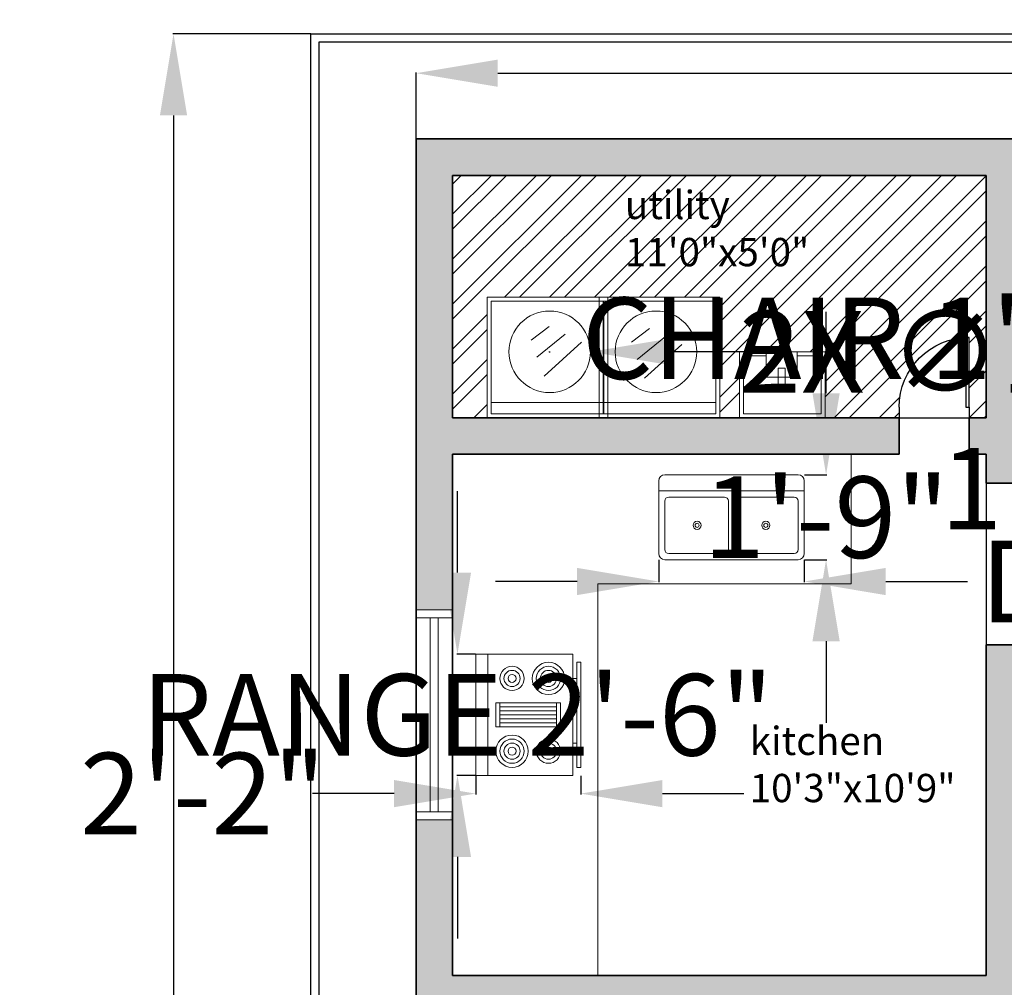
# Model space of a CAD drawing. Units: inches. Extents: x 1202 to 2101, y 998 to 1743.
# Tile 2 of 4: x 1310 to 1553, y 1460 to 1699. Entities that reach past the tile are written whole.
import ezdxf

# ---------------------------------------------------------------- set-up
doc = ezdxf.new("R2010")
doc.units = ezdxf.units.IN
doc.header["$MEASUREMENT"] = 0
for name, color, linetype, lineweight in [('A-ANNO-DIMS', 2, 'Continuous', 18), ('A-AREA-IDEN', 7, 'Continuous', 18), ('A-DOOR', 3, 'Continuous', 25), ('A-EQPM', 8, 'Continuous', 18), ('A-FLOR-CASE', 8, 'Continuous', 18), ('A-FLOR-FIXT', 9, 'Continuous', 18), ('A-FLOR-PATT', 9, 'Continuous', 13), ('A-GLAZ', 4, 'Continuous', 18), ('A-WALL', 7, 'Continuous', 35), ('A-WALL-PATT', 250, 'Continuous', 13), ('C-PROP', 7, 'Continuous', 30)]:
    doc.layers.add(name, color=color, linetype=linetype, lineweight=lineweight)
doc.styles.get("Standard").update_dxf_attribs({"font": 'arial.ttf'})
doc.dimstyles.get("Standard").update_dxf_attribs({"dimtxt": 20.18, "dimasz": 20.18, "dimexe": 0.18, "dimexo": 0.0625, "dimgap": 0.09, "dimtad": 0, "dimtih": 1, "dimtoh": 1, "dimdec": 0, "dimzin": 0, "dimdsep": 46, "dimlunit": 3, "dimtxsty": 'Standard', "dimcen": 0.09, "dimadec": 0, "dimazin": 0, "dimtfac": 1, "dimtdec": 0, "dimtofl": 0, "dimtmove": 0, "dimatfit": 3, "dimfxl": 1, "dimtolj": 1, "dimtzin": 0, "dimarcsym": 0})

# ---------------------------------------------------------------- blocks, each defined once
blk = doc.blocks.new('*U2')
for p, q in [((0, 0), (0, -6)), ((40, 0), (40, -6))]:
    blk.add_line(p, q)
blk.add_lwpolyline([(0, 0), (0, 40), (1.75, 40), (1.75, 0)], close=True)
blk.add_arc((0, 0), 40, 0, 90)
blk = doc.blocks.new('Range-Oven - 30 in top')
for p, q in [((0, -3), (30, -3)), ((12, -6), (18, -6)), ((13, -20), (13, -6)), ((14, -6), (14, -20)), ((15, -20), (15, -6)), ((16, -6), (16, -20)), ((17, -20), (17, -6)), ((18, -20), (12, -20)), ((6, -24), (6, -25)), ((8, -25), (8, -24)), ((22, -25), (22, -24)), ((24, -24), (24, -25))]:
    blk.add_line(p, q)
for points in [[(0, -24), (0, 0), (30, 0), (30, -24)], [(12, -21), (12, -5), (18, -5), (18, -21)], [(2, -26), (2, -25), (28, -25), (28, -26)]]:
    blk.add_lwpolyline(points, close=True)
for centre, radius in [((6, -9), 4), ((6, -9), 3), ((6, -9), 2), ((24, -9), 3), ((24, -9), 2), ((6, -9), 1), ((24, -9), 1), ((24, -18), 4), ((6, -18), 3), ((6, -18), 2), ((6, -18), 1), ((24, -18), 3), ((24, -18), 2), ((24, -18), 1)]:
    blk.add_circle(centre, radius)
blk = doc.blocks.new('Sink-double - 36 in top')
for p, q in [((-18, -4), (18, -4)), ((-0.75, -18.5), (-0.75, -6.5)), ((0.75, -6.5), (0.75, -18.5))]:
    blk.add_line(p, q)
for points in [[(-16.5, 0), (16.5, 0)], [(-18, -19.5), (-18, -1.5)], [(18, -1.5), (18, -19.5)], [(-16.5, -18.5), (-16.5, -6.5)], [(-15.5, -5.5), (-1.75, -5.5)], [(1.75, -5.5), (15.5, -5.5)], [(16.5, -6.5), (16.5, -18.5)], [(16.5, -21), (-16.5, -21)], [(-1.75, -19.5), (-15.5, -19.5)], [(15.5, -19.5), (1.75, -19.5)]]:
    blk.add_lwpolyline(points)
for centre, radius in [((-8.5, -12.5), 1), ((-8.5, -12.5), 0.5), ((8.5, -12.5), 1), ((8.5, -12.5), 0.5)]:
    blk.add_circle(centre, radius)
for centre, radius, start, end in [((-16.5, -1.5), 1.5, 90, 180), ((16.5, -1.5), 1.5, 0, 90), ((-15.5, -6.5), 1, 90, 180), ((-1.75, -6.5), 1, 0, 90), ((1.75, -6.5), 1, 90, 180), ((15.5, -6.5), 1, 0, 90), ((-15.5, -18.5), 1, 180, 270), ((-1.75, -18.5), 1, 270, 0), ((1.75, -18.5), 1, 180, 270), ((15.5, -18.5), 1, 270, 0), ((-16.5, -19.5), 1.5, 180, 270), ((16.5, -19.5), 1.5, 270, 0)]:
    blk.add_arc(centre, radius, start, end)
blk = doc.blocks.new('*D9')
at = {"layer": 'A-ANNO-DIMS', "color": 0, "lineweight": -2, "transparency": 16777216}
for p, q in [((1407.98, 1669.53), (1407.98, 1685.93)), ((1428.16, 1685.75), (1570.77, 1685.75)), ((1747.8, 1685.75), (1605.18, 1685.75)), ((1767.98, 1669.53), (1767.98, 1685.93))]:
    blk.add_line(p, q, dxfattribs=at)
at = {"layer": 'A-ANNO-DIMS', "color": 0, "transparency": 16777216}
for points in [[(1428.16, 1689.11), (1428.16, 1682.38), (1407.98, 1685.75)], [(1747.8, 1689.11), (1747.8, 1682.38), (1767.98, 1685.75)]]:
    blk.add_solid(points, dxfattribs=at)
at = {"layer": 'Defpoints', "color": 0, "transparency": 16777216}
for p in [(1767.98, 1685.75), (1407.98, 1669.47), (1767.98, 1669.47)]:
    blk.add_point(p, dxfattribs=at)
at = {"layer": 'A-ANNO-DIMS', "color": 0, "transparency": 16777216, "insert": (1587.98, 1685.75), "char_height": 20.18, "attachment_point": 5}
blk.add_mtext("\\A1;30'", dxfattribs=at)
blk = doc.blocks.new('WIN-48IN-PLAN')
for p, q in [((9, 48), (0, 48)), ((3.5, 48), (3.5, 0)), ((5.5, 48), (5.5, 0)), ((9, 0), (0, 0))]:
    blk.add_line(p, q)
blk = doc.blocks.new('*D31')
at = {"layer": 'A-ANNO-DIMS', "color": 0, "lineweight": -2, "transparency": 16777216}
for p, q in [((1418.22, 1562.15), (1418.22, 1582.33)), ((1422.65, 1541.97), (1418.04, 1541.97)), ((1422.65, 1511.97), (1418.04, 1511.97)), ((1418.22, 1491.79), (1418.22, 1471.61))]:
    blk.add_line(p, q, dxfattribs=at)
at = {"layer": 'A-ANNO-DIMS', "color": 0, "transparency": 16777216}
for points in [[(1414.85, 1562.15), (1421.58, 1562.15), (1418.22, 1541.97)], [(1414.85, 1491.79), (1421.58, 1491.79), (1418.22, 1511.97)]]:
    blk.add_solid(points, dxfattribs=at)
at = {"layer": 'Defpoints', "color": 0, "transparency": 16777216}
for p in [(1418.22, 1541.97), (1422.72, 1541.97), (1422.72, 1511.97)]:
    blk.add_point(p, dxfattribs=at)
at = {"layer": 'A-ANNO-DIMS', "color": 0, "transparency": 16777216, "insert": (1418.22, 1526.97), "char_height": 20.18, "attachment_point": 5}
blk.add_mtext('\\A1;RANGE 2\'-6"', dxfattribs=at)
blk = doc.blocks.new('*D32')
at = {"layer": 'A-ANNO-DIMS', "color": 0, "lineweight": -2, "transparency": 16777216}
for p, q in [((1422.72, 1511.9), (1422.72, 1507.29)), ((1448.72, 1511.9), (1448.72, 1507.29)), ((1402.54, 1507.47), (1382.36, 1507.47)), ((1468.9, 1507.47), (1489.08, 1507.47))]:
    blk.add_line(p, q, dxfattribs=at)
at = {"layer": 'A-ANNO-DIMS', "color": 0, "transparency": 16777216}
for points in [[(1402.54, 1510.83), (1402.54, 1504.1), (1422.72, 1507.47)], [(1468.9, 1510.83), (1468.9, 1504.1), (1448.72, 1507.47)]]:
    blk.add_solid(points, dxfattribs=at)
at = {"layer": 'Defpoints', "color": 0, "transparency": 16777216}
for p in [(1422.72, 1511.97), (1448.72, 1511.97), (1422.72, 1507.47)]:
    blk.add_point(p, dxfattribs=at)
at = {"layer": 'A-ANNO-DIMS', "color": 0, "transparency": 16777216, "insert": (1355.27, 1507.47), "char_height": 20.18, "attachment_point": 5}
blk.add_mtext('\\A1;2\'-2"', dxfattribs=at)
blk = doc.blocks.new('*D33')
at = {"layer": 'A-ANNO-DIMS', "color": 0, "lineweight": -2, "transparency": 16777216}
for p, q in [((1467.99, 1565.29), (1467.99, 1559.78)), ((1503.99, 1565.29), (1503.99, 1559.78)), ((1447.81, 1559.96), (1427.63, 1559.96)), ((1524.17, 1559.96), (1544.35, 1559.96))]:
    blk.add_line(p, q, dxfattribs=at)
at = {"layer": 'A-ANNO-DIMS', "color": 0, "transparency": 16777216}
for points in [[(1447.81, 1563.32), (1447.81, 1556.59), (1467.99, 1559.96)], [(1524.17, 1563.32), (1524.17, 1556.59), (1503.99, 1559.96)]]:
    blk.add_solid(points, dxfattribs=at)
at = {"layer": 'Defpoints', "color": 0, "transparency": 16777216}
for p in [(1467.99, 1565.36), (1503.99, 1565.36), (1503.99, 1559.96)]:
    blk.add_point(p, dxfattribs=at)
at = {"layer": 'A-ANNO-DIMS', "color": 0, "transparency": 16777216, "insert": (1669.46, 1559.96), "char_height": 20.18, "attachment_point": 5}
blk.add_mtext('\\A1;DOUBLE SINK 3\'-0"', dxfattribs=at)
blk = doc.blocks.new('*D34')
at = {"layer": 'A-ANNO-DIMS', "color": 0, "lineweight": -2, "transparency": 16777216}
for p, q in [((1509.39, 1606.54), (1509.39, 1626.72)), ((1504.05, 1586.36), (1509.57, 1586.36)), ((1504.05, 1565.36), (1509.57, 1565.36)), ((1509.39, 1545.18), (1509.39, 1525))]:
    blk.add_line(p, q, dxfattribs=at)
at = {"layer": 'A-ANNO-DIMS', "color": 0, "transparency": 16777216}
for points in [[(1506.03, 1606.54), (1512.76, 1606.54), (1509.39, 1586.36)], [(1506.03, 1545.18), (1512.76, 1545.18), (1509.39, 1565.36)]]:
    blk.add_solid(points, dxfattribs=at)
at = {"layer": 'Defpoints', "color": 0, "transparency": 16777216}
for p in [(1503.99, 1586.36), (1509.39, 1586.36), (1503.99, 1565.36)]:
    blk.add_point(p, dxfattribs=at)
at = {"layer": 'A-ANNO-DIMS', "color": 0, "transparency": 16777216, "insert": (1509.39, 1575.86), "char_height": 20.18, "attachment_point": 5}
blk.add_mtext('\\A1;1\'-9"', dxfattribs=at)
blk = doc.blocks.new('*D35')
at = {"layer": 'A-ANNO-DIMS', "color": 0, "lineweight": -2, "transparency": 16777216}
for p, q in [((1637.33, 1623.23), (1637.33, 1619.96)), ((1658.33, 1623.23), (1658.33, 1619.96)), ((1617.15, 1620.14), (1596.97, 1620.14)), ((1678.51, 1620.14), (1698.69, 1620.14))]:
    blk.add_line(p, q, dxfattribs=at)
at = {"layer": 'A-ANNO-DIMS', "color": 0, "transparency": 16777216}
for points in [[(1617.15, 1623.51), (1617.15, 1616.78), (1637.33, 1620.14)], [(1678.51, 1623.51), (1678.51, 1616.78), (1658.33, 1620.14)]]:
    blk.add_solid(points, dxfattribs=at)
at = {"layer": 'Defpoints', "color": 0, "transparency": 16777216}
for p in [(1637.33, 1623.29), (1658.33, 1623.29), (1637.33, 1620.14)]:
    blk.add_point(p, dxfattribs=at)
at = {"layer": 'A-ANNO-DIMS', "color": 0, "transparency": 16777216, "insert": (1522.41, 1620.14), "char_height": 20.18, "attachment_point": 5}
blk.add_mtext('\\A1;CHAIR 1\'-9"', dxfattribs=at)
blk = doc.blocks.new('*D36')
at = {"layer": 'A-ANNO-DIMS', "color": 0, "lineweight": -2, "transparency": 16777216}
for p, q in [((1661.48, 1660.81), (1661.48, 1680.99)), ((1658.4, 1640.63), (1661.66, 1640.63)), ((1658.4, 1623.29), (1661.66, 1623.29)), ((1661.48, 1603.11), (1661.48, 1582.93)), ((1661.48, 1582.93), (1641.3, 1582.93))]:
    blk.add_line(p, q, dxfattribs=at)
at = {"layer": 'A-ANNO-DIMS', "color": 0, "transparency": 16777216}
for points in [[(1658.12, 1660.81), (1664.85, 1660.81), (1661.48, 1640.63)], [(1658.12, 1603.11), (1664.85, 1603.11), (1661.48, 1623.29)]]:
    blk.add_solid(points, dxfattribs=at)
at = {"layer": 'Defpoints', "color": 0, "transparency": 16777216}
for p in [(1658.33, 1640.63), (1658.33, 1623.29), (1661.48, 1623.29)]:
    blk.add_point(p, dxfattribs=at)
at = {"layer": 'A-ANNO-DIMS', "color": 0, "transparency": 16777216, "insert": (1591.83, 1582.93), "char_height": 20.18, "attachment_point": 5}
blk.add_mtext('\\A1;1\'-5 1/2"', dxfattribs=at)
blk = doc.blocks.new('*D40')
at = {"layer": 'A-ANNO-DIMS', "color": 0, "lineweight": -2, "transparency": 16777216}
for p, q in [((1381.91, 1695.47), (1347.8, 1695.47)), ((1347.98, 1675.29), (1347.98, 1380.86)), ((1347.98, 1065.65), (1347.98, 1360.07)), ((1381.91, 1045.47), (1347.8, 1045.47))]:
    blk.add_line(p, q, dxfattribs=at)
at = {"layer": 'A-ANNO-DIMS', "color": 0, "transparency": 16777216}
for points in [[(1344.61, 1675.29), (1351.34, 1675.29), (1347.98, 1695.47)], [(1344.61, 1065.65), (1351.34, 1065.65), (1347.98, 1045.47)]]:
    blk.add_solid(points, dxfattribs=at)
at = {"layer": 'Defpoints', "color": 0, "transparency": 16777216}
for p in [(1347.98, 1695.47), (1381.98, 1695.47), (1381.98, 1045.47)]:
    blk.add_point(p, dxfattribs=at)
at = {"layer": 'A-ANNO-DIMS', "color": 0, "transparency": 16777216, "insert": (1347.98, 1370.47), "char_height": 20.18, "attachment_point": 5}
blk.add_mtext('\\A1;54\'-2"', dxfattribs=at)
blk = doc.blocks.new('*D51')
at = {"layer": 'A-ANNO-DIMS', "color": 0, "lineweight": -2, "transparency": 16777216}
for p, q in [((1440.93, 1616.8), (1441.11, 1616.8)), ((1441.02, 1616.71), (1441.02, 1616.89)), ((1491.46, 1616.8), (1471.28, 1616.8))]:
    blk.add_line(p, q, dxfattribs=at)
at = {"layer": 'A-ANNO-DIMS', "color": 0, "transparency": 16777216}
blk.add_solid([(1471.28, 1620.16), (1471.28, 1613.43), (1451.1, 1616.8)], dxfattribs=at)
at = {"layer": 'Defpoints', "color": 0, "transparency": 16777216}
for p in [(1430.93, 1616.8), (1451.1, 1616.8)]:
    blk.add_point(p, dxfattribs=at)
at = {"layer": 'A-ANNO-DIMS', "color": 0, "transparency": 16777216, "insert": (1550.67, 1616.8), "char_height": 20.18, "attachment_point": 5}
blk.add_mtext('\\A1;2X ∅1\'-8"', dxfattribs=at)

msp = doc.modelspace()

# ---------------------------------------------------------------- hatches: boundary and pattern name
at = {"layer": 'A-FLOR-PATT'}
h = msp.add_hatch(dxfattribs=at)
h.set_pattern_fill('ANSI32', color=256, scale=21)
h.paths.add_polyline_path([(1548.98, 1660.47), (1416.98, 1660.47), (1416.98, 1600.47), (1425.57, 1600.47), (1425.57, 1630.31), (1455.41, 1630.31), (1483.1, 1630.31), (1483.1, 1600.47), (1487.96, 1600.47), (1487.96, 1616.8), (1509.17, 1616.8), (1509.17, 1600.47), (1527.46, 1600.47), (1527.46, 1603.06, -0.401453), (1544, 1620.33), (1544, 1620.35), (1544.75, 1620.35), (1544.75, 1603.06), (1544.75, 1600.47), (1548.98, 1600.47)])
at = {"layer": 'A-WALL-PATT'}
h = msp.add_hatch(color=256, dxfattribs=at)
h.dxf.hatch_style = 1
h.paths.add_polyline_path([(1767.98, 1669.47), (1407.98, 1669.47), (1407.98, 1552.97), (1416.98, 1552.97), (1416.98, 1591.47), (1527.46, 1591.47), (1527.46, 1600.47), (1416.98, 1600.47), (1416.98, 1660.47), (1548.98, 1660.47), (1548.98, 1600.47), (1544.75, 1600.47), (1544.75, 1591.47), (1548.98, 1591.47), (1548.98, 1584.29), (1557.98, 1584.29), (1557.98, 1660.47), (1617.98, 1660.47), (1617.98, 1540.47), (1557.98, 1540.47), (1557.98, 1544.29), (1548.98, 1544.29), (1548.98, 1462.47), (1416.98, 1462.47), (1416.98, 1500.97), (1407.98, 1500.97), (1407.98, 1424.63), (1416.98, 1424.63), (1416.98, 1431.74), (1416.98, 1453.47), (1557.98, 1453.47), (1557.98, 1531.47), (1617.98, 1531.47), (1617.98, 1507.47), (1622.48, 1507.47, -0.014283), (1624.48, 1507.47), (1626.98, 1507.47), (1626.98, 1660.47), (1758.98, 1660.47), (1758.98, 1638.32), (1758.98, 1561.97), (1767.98, 1561.97)])
h.paths.add_polyline_path([(1416.98, 1372.63), (1407.98, 1372.63), (1407.98, 1318.84), (1416.98, 1318.84)])
h.paths.add_polyline_path([(1626.98, 1390.47), (1758.98, 1390.47), (1758.98, 1369.1), (1758.98, 1344.47), (1767.98, 1344.47), (1767.98, 1415.47), (1758.98, 1415.47), (1758.98, 1399.47), (1680.98, 1399.47), (1680.98, 1425.58), (1671.98, 1425.58), (1671.98, 1399.47), (1626.98, 1399.47), (1626.98, 1459.47), (1631.88, 1459.47), (1631.88, 1461.58), (1631.88, 1468.47), (1626.98, 1468.47), (1626.98, 1471.47), (1622.48, 1471.47), (1617.98, 1471.47), (1617.98, 1261.47), (1614.74, 1261.47), (1614.74, 1258.47), (1614.74, 1252.47), (1617.98, 1252.47), (1617.98, 1144.47), (1758.98, 1144.47), (1758.98, 1125.47), (1767.98, 1125.47), (1767.98, 1169.47), (1758.98, 1169.47), (1758.98, 1153.47), (1680.98, 1153.47), (1680.98, 1179.68, -0.04329), (1676.17, 1179.26), (1671.98, 1179.26), (1671.98, 1153.47), (1626.98, 1153.47), (1626.98, 1213.47), (1631.88, 1213.47), (1631.88, 1218.24), (1631.88, 1222.47), (1626.98, 1222.47)])
h.paths.add_polyline_path([(1767.98, 1509.97), (1758.98, 1509.97), (1758.98, 1468.47), (1660.05, 1468.47), (1660.05, 1461.58), (1660.05, 1459.47), (1671.98, 1459.47), (1671.98, 1453.51), (1680.98, 1453.51), (1680.98, 1459.47), (1758.98, 1459.47), (1758.98, 1443.47), (1767.98, 1443.47)], flags=17)
h.paths.add_polyline_path([(1767.98, 1268.47), (1758.98, 1268.47), (1758.98, 1263.28), (1758.98, 1222.47), (1660.05, 1222.47), (1660.05, 1218.24, -0.04262), (1659.64, 1213.47), (1671.98, 1213.47), (1671.98, 1207.19), (1676.17, 1207.19), (1680.98, 1207.19), (1680.98, 1213.47), (1758.98, 1213.47), (1758.98, 1197.47), (1767.98, 1197.47)], flags=17)
h.paths.add_polyline_path([(1767.98, 1073.47), (1758.98, 1073.47), (1758.98, 1054.47), (1767.98, 1054.47)])

# ---------------------------------------------------------------- linework, layer by layer
at = {"layer": 'A-DOOR'}
for p, q in [((1527.46, 1600.47), (1544.75, 1600.47)), ((1548.98, 1584.29), (1548.98, 1544.29))]:
    msp.add_line(p, q, dxfattribs=at)
at = {"layer": 'A-EQPM'}
for p, q in [((1436.41, 1619.71), (1440.87, 1623.09)), ((1461.24, 1619.18), (1465.7, 1622.56)), ((1437.84, 1615.44), (1444.88, 1621.13)), ((1462.67, 1614.9), (1469.71, 1620.6)), ((1439.62, 1610.81), (1448.89, 1619.18)), ((1464.45, 1610.27), (1473.72, 1618.64)), ((1426.57, 1604.23), (1482.1, 1604.23))]:
    msp.add_line(p, q, dxfattribs=at)
for points in [[(1425.57, 1630.31), (1455.41, 1630.31), (1455.41, 1600.47), (1425.57, 1600.47)], [(1453.26, 1630.31), (1483.1, 1630.31), (1483.1, 1600.47), (1453.26, 1600.47)], [(1426.57, 1629.31), (1454.41, 1629.31), (1454.41, 1601.47), (1426.57, 1601.47)], [(1454.26, 1629.31), (1482.1, 1629.31), (1482.1, 1601.47), (1454.26, 1601.47)], [(1454.26, 1629.31), (1482.1, 1629.31), (1482.1, 1601.47), (1454.26, 1601.47)]]:
    msp.add_lwpolyline(points, close=True, dxfattribs=at)
for centre in [(1441.02, 1616.8), (1467.31, 1616.8)]:
    msp.add_circle(centre, 10.09, dxfattribs=at)
at = {"layer": 'A-FLOR-CASE'}
for p, q in [((1515.62, 1591.47), (1515.62, 1559.41)), ((1515.62, 1559.41), (1452.94, 1559.41)), ((1452.94, 1559.41), (1452.94, 1462.47))]:
    msp.add_line(p, q, dxfattribs=at)
at = {"layer": 'A-FLOR-FIXT'}
for p, q in [((1499.24, 1612.72), (1497.57, 1612.72)), ((1497.57, 1612.72), (1497.57, 1607.85)), ((1499.24, 1607.94), (1499.24, 1612.72)), ((1499.24, 1612.72), (1499.24, 1612.72)), ((1497.57, 1607.85), (1499.24, 1607.85))]:
    msp.add_line(p, q, dxfattribs=at)
for points in [[(1487.96, 1616.8), (1509.17, 1616.8), (1509.17, 1600.47), (1487.96, 1600.47)], [(1494.57, 1616.8), (1502.24, 1616.8), (1502.24, 1610.56), (1494.57, 1610.56)]]:
    msp.add_lwpolyline(points, close=True, dxfattribs=at)
msp.add_lwpolyline([(1502.24, 1615.8), (1508.17, 1615.8), (1508.17, 1601.47), (1488.96, 1601.47), (1488.96, 1615.8), (1494.57, 1615.8)], dxfattribs=at)
at = {"layer": 'A-GLAZ'}
for p, q in [((1416.98, 1552.97), (1407.98, 1552.97)), ((1413.48, 1550.97), (1413.48, 1502.97)), ((1416.98, 1500.97), (1407.98, 1500.97))]:
    msp.add_line(p, q, dxfattribs=at)
at = {"layer": 'A-WALL'}
for p, q in [((1407.98, 1252.47), (1407.98, 1669.47)), ((1407.98, 1669.47), (1767.98, 1669.47)), ((1416.98, 1660.47), (1548.98, 1660.47)), ((1416.98, 1600.47), (1416.98, 1660.47)), ((1548.98, 1600.47), (1548.98, 1660.47)), ((1416.98, 1600.47), (1527.46, 1600.47)), ((1527.46, 1600.47), (1527.46, 1591.47)), ((1544.75, 1600.47), (1544.75, 1591.47)), ((1544.75, 1600.47), (1548.98, 1600.47)), ((1416.98, 1591.47), (1527.46, 1591.47)), ((1416.98, 1462.47), (1416.98, 1591.47)), ((1544.75, 1591.47), (1548.98, 1591.47)), ((1548.98, 1584.29), (1548.98, 1591.47)), ((1557.98, 1584.29), (1548.98, 1584.29)), ((1548.98, 1462.47), (1548.98, 1544.29)), ((1557.98, 1544.29), (1548.98, 1544.29)), ((1416.98, 1462.47), (1548.98, 1462.47))]:
    msp.add_line(p, q, dxfattribs=at)
at = {"layer": 'C-PROP'}
for p, q in [((1381.98, 1045.47), (1381.98, 1695.47)), ((1381.98, 1695.47), (1793.98, 1695.47)), ((1383.98, 1693.47), (1791.98, 1693.47)), ((1383.98, 1054.47), (1383.98, 1693.47))]:
    msp.add_line(p, q, dxfattribs=at)

# ---------------------------------------------------------------- block references
at = {"layer": 'A-DOOR', "xscale": -0.4321919262010457, "yscale": 0.4321919262010457, "zscale": 0.4321919262010457}
msp.add_blockref('*U2', (1544.75, 1603.06), dxfattribs=at)
at = {"layer": 'A-EQPM', "rotation": 89.99999999999999}
msp.add_blockref('Range-Oven - 30 in top', (1422.72, 1511.97), dxfattribs=at)
at = {"layer": 'A-FLOR-FIXT'}
msp.add_blockref('Sink-double - 36 in top', (1485.99, 1586.36), dxfattribs=at)
at = {"layer": 'A-GLAZ'}
msp.add_blockref('WIN-48IN-PLAN', (1407.98, 1502.97), dxfattribs=at)

# ---------------------------------------------------------------- texts
at = {"layer": 'A-AREA-IDEN', "char_height": 7, "attachment_point": 1}
for s, insert in [('utility\\P11\'0"x5\'0"', (1459.63, 1656.64)), ('kitchen\\P10\'3"x10\'9"', (1490.5, 1524.02))]:
    msp.add_mtext_dynamic_manual_height_columns(s, width=28.6147, gutter_width=1, heights=[0], dxfattribs=dict(at, insert=insert))

# ---------------------------------------------------------------- dimensions: what is measured, and where the dimension line sits
at = {"layer": 'A-ANNO-DIMS'}
dim = msp.add_linear_dim(base=(1767.98, 1685.75), p1=(1407.98, 1669.47), p2=(1767.98, 1669.47), dimstyle='Standard', override={"dimclrd": 0, "dimclre": 0, "dimclrt": 0}, dxfattribs=at)
dim.commit()
dim.dimension.update_dxf_attribs({"geometry": '*D9', "text_midpoint": (1587.98, 1685.75)})
for base, p1, p2, angle, picture, middle in [((1347.98, 1695.47), (1381.98, 1045.47), (1381.98, 1695.47), 90, '*D40', (1347.98, 1370.47)), ((1661.48, 1623.29), (1658.33, 1640.63), (1658.33, 1623.29), 270, '*D36', (1591.83, 1582.93)), ((1509.39, 1586.36), (1503.99, 1565.36), (1503.99, 1586.36), 90, '*D34', (1509.39, 1575.86)), ((1422.72, 1507.47), (1448.72, 1511.97), (1422.72, 1511.97), 180, '*D32', (1355.27, 1507.47))]:
    dim = msp.add_linear_dim(base=base, p1=p1, p2=p2, angle=angle, dimstyle='Standard', override={"dimdec": 1, "dimlfac": 1, "dimrnd": 0, "dimzin": 1, "dimdsep": 46, "dimlunit": 4, "dimfrac": 2}, dxfattribs=at)
    dim.commit()
    dim.dimension.update_dxf_attribs({"geometry": picture, "text_midpoint": middle})
for base, p1, p2, angle, text, picture, middle in [((1637.33, 1620.14), (1658.33, 1623.29), (1637.33, 1623.29), 180, 'CHAIR <>', '*D35', (1522.41, 1620.14)), ((1418.22, 1541.97), (1422.72, 1511.97), (1422.72, 1541.97), 90, 'RANGE <>', '*D31', (1418.22, 1526.97))]:
    dim = msp.add_linear_dim(base=base, p1=p1, p2=p2, angle=angle, text=text, dimstyle='Standard', override={"dimdec": 1, "dimlfac": 1, "dimrnd": 0, "dimzin": 1, "dimdsep": 46, "dimlunit": 4, "dimfrac": 2}, dxfattribs=at)
    dim.commit()
    dim.dimension.update_dxf_attribs({"geometry": picture, "text_midpoint": middle})
dim = msp.add_diameter_dim_2p(p1=(1430.93, 1616.8), p2=(1451.1, 1616.8), text='2X <>', dimstyle='Standard', override={"dimdec": 1, "dimlfac": 1, "dimrnd": 0, "dimzin": 1, "dimdsep": 46, "dimlunit": 4, "dimfrac": 2}, dxfattribs=at)
dim.commit()
dim.dimension.update_dxf_attribs({"geometry": '*D51', "text_midpoint": (1491.46, 1616.8)})
dim = msp.add_linear_dim(base=(1503.99, 1559.96), p1=(1467.99, 1565.36), p2=(1503.99, 1565.36), text='DOUBLE SINK <>', dimstyle='Standard', override={"dimdec": 1, "dimlfac": 1, "dimrnd": 0, "dimzin": 1, "dimdsep": 46, "dimlunit": 4, "dimfrac": 2}, dxfattribs=at)
dim.commit()
dim.dimension.update_dxf_attribs({"geometry": '*D33', "text_midpoint": (1669.46, 1559.96)})

doc.saveas('drawing.dxf')
